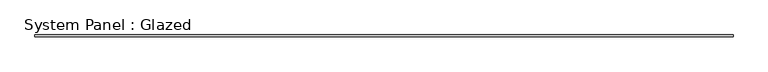
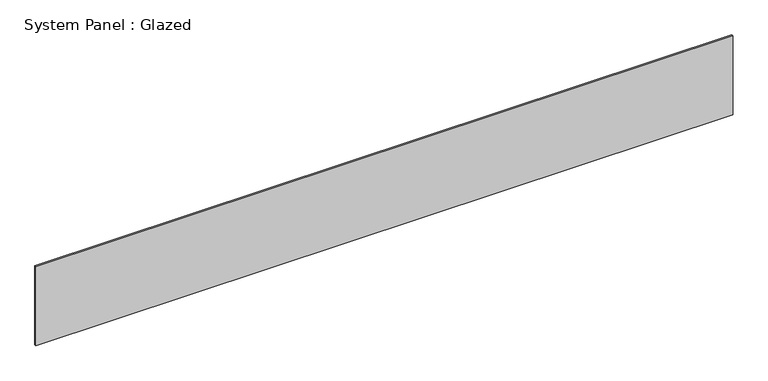
"""IFC4 building model written with IfcOpenShell, lengths in millimetres: plate geometry, System Panel : Glazed."""

from ifc_helpers import new_model, si_unit, origin, origin_with_axes, place, context, project, spatial, polyline, outline, extrude, source, transform, mapped, element, save


def system_panel_glazed_144e3648(model_context):
    return source(origin(), model_context, "Body", "SweptSolid", [
        extrude(outline(polyline([(5094.544138, 19.05), (-5094.544138, 19.05), (-5094.544138, 44.45), (5094.544138, 44.45), (5094.544138, 19.05)])), origin_with_axes(), (0.0, 0.0, 1.0), 1219.2),
    ])


if __name__ == "__main__":
    model = new_model("IFC4")
    model_context = context("Model", 3, world=origin())
    ifc_project = project(units=[si_unit("LENGTHUNIT", "METRE", prefix="MILLI")], contexts=[model_context])
    site = spatial("IfcSite", under=ifc_project)
    building = spatial("IfcBuilding", under=site)
    placement = place(None, origin())
    system_panel_glazed_shape = system_panel_glazed_144e3648(model_context)
    element("IfcPlate", 1, ObjectType="System Panel : Glazed", at=placement, inside=building, context=model_context, shape_type="MappedRepresentation", body=[
        mapped(system_panel_glazed_shape, transform((0.0, 0.0, 0.0), x_axis=(1.0, 0.0, 0.0), y_axis=(0.0, 1.0, 0.0), z_axis=(0.0, 0.0, 1.0))),
    ])
    save(model, "model.ifc")

# Revit data of these elements
# Type "System Panel : Glazed"
#   Construction Type Id = "GSP4R"
#   Analytic Construction = "1/8 in Pilkington single glazing"
#   Visual Light Transmittance = 0.9
#   Solar Heat Gain Coefficient = 0.86
#   Heat Transfer Coefficient (U) = 1.18115 BTU/(h·ft²·°F)
# Element 1 (IfcPlate, "System Panel : Glazed")
#   Materials on its faces: "Glass"
# Materials
#   "Glass": class "Glass", colour RGB 0 128 192, transparency 0.75, Description = "Soda Lime Glass", Cost = 0
